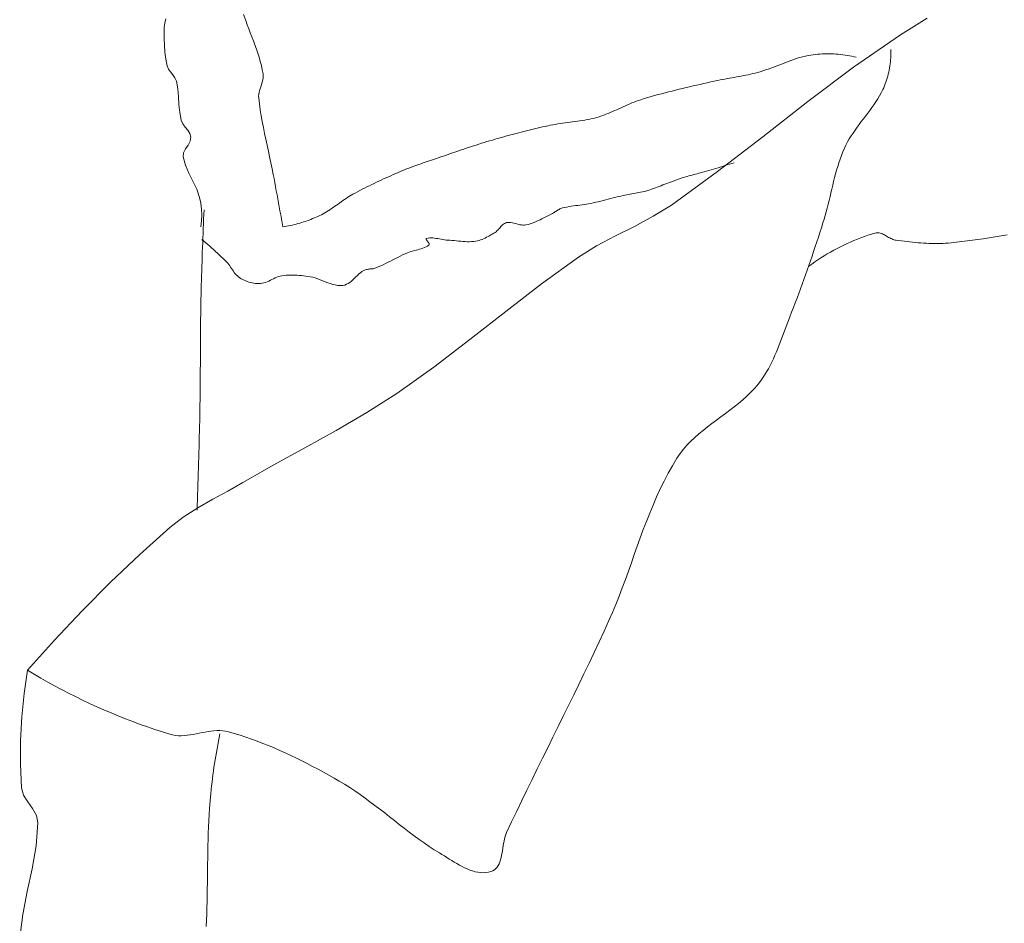
# Model space of a CAD drawing. Units: inches. Extents: x -36302355 to 648, y -221479757 to 75.
# Tile 25 of 37: x 192 to 220, y -218 to -192. Entities that reach past the tile are written whole.
import ezdxf

# ---------------------------------------------------------------- set-up
doc = ezdxf.new("R2010")
doc.units = ezdxf.units.IN
doc.header["$MEASUREMENT"] = 0
doc.layers.add('A-FURN', color=8, linetype='Continuous', lineweight=13)

# ---------------------------------------------------------------- blocks, each defined once
blk = doc.blocks.new('BED-DOUBLE')
for p, q in [((4.097, 63.43), (4.117, 63.548)), ((6.36, 63.496), (6.296, 63.67)), ((6.401, 63.383), (6.36, 63.496)), ((25.45, 63.569), (24.695, 63.097)), ((4.072, 63.192), (4.078, 63.311)), ((4.076, 62.999), (4.072, 63.192)), ((4.078, 63.311), (4.097, 63.43)), ((6.444, 63.269), (6.401, 63.383)), ((6.488, 63.156), (6.444, 63.269)), ((6.531, 63.043), (6.488, 63.156)), ((4.083, 62.806), (4.076, 62.999)), ((6.574, 62.929), (6.531, 63.043)), ((6.616, 62.816), (6.574, 62.929)), ((24.695, 63.097), (23.379, 62.192)), ((4.096, 62.613), (4.083, 62.806)), ((4.119, 62.421), (4.096, 62.613)), ((6.657, 62.702), (6.616, 62.816)), ((6.696, 62.587), (6.657, 62.702)), ((24.428, 62.63), (24.425, 62.688)), ((24.428, 62.573), (24.428, 62.63)), ((4.157, 62.233), (4.119, 62.421)), ((6.733, 62.472), (6.696, 62.587)), ((6.767, 62.356), (6.733, 62.472)), ((6.797, 62.24), (6.767, 62.356)), ((21.511, 62.338), (21.437, 62.31)), ((21.585, 62.366), (21.511, 62.338)), ((21.659, 62.392), (21.585, 62.366)), ((21.733, 62.418), (21.659, 62.392)), ((21.808, 62.442), (21.733, 62.418)), ((21.883, 62.464), (21.808, 62.442)), ((21.958, 62.485), (21.883, 62.464)), ((22.034, 62.503), (21.958, 62.485)), ((22.111, 62.519), (22.034, 62.503)), ((22.188, 62.532), (22.111, 62.519)), ((22.251, 62.541), (22.188, 62.532)), ((22.315, 62.549), (22.251, 62.541)), ((22.378, 62.555), (22.315, 62.549)), ((22.442, 62.561), (22.378, 62.555)), ((22.506, 62.564), (22.442, 62.561)), ((22.57, 62.567), (22.506, 62.564)), ((22.635, 62.568), (22.57, 62.567)), ((22.699, 62.568), (22.635, 62.568)), ((22.763, 62.567), (22.699, 62.568)), ((22.828, 62.565), (22.763, 62.567)), ((22.892, 62.561), (22.828, 62.565)), ((22.956, 62.556), (22.892, 62.561)), ((23.02, 62.55), (22.956, 62.556)), ((23.084, 62.542), (23.02, 62.55)), ((23.148, 62.533), (23.084, 62.542)), ((23.211, 62.523), (23.148, 62.533)), ((23.274, 62.512), (23.211, 62.523)), ((23.337, 62.499), (23.274, 62.512)), ((23.399, 62.485), (23.337, 62.499)), ((23.461, 62.47), (23.399, 62.485)), ((24.41, 62.285), (24.417, 62.342)), ((24.417, 62.342), (24.422, 62.4)), ((24.422, 62.4), (24.425, 62.458)), ((24.425, 62.458), (24.428, 62.515)), ((24.428, 62.515), (24.428, 62.573)), ((4.195, 62.142), (4.157, 62.233)), ((4.253, 62.059), (4.195, 62.142)), ((4.318, 61.979), (4.253, 62.059)), ((6.824, 62.122), (6.797, 62.24)), ((6.846, 62.004), (6.824, 62.122)), ((20.771, 62.067), (20.695, 62.046)), ((20.846, 62.09), (20.771, 62.067)), ((20.921, 62.115), (20.846, 62.09)), ((20.995, 62.141), (20.921, 62.115)), ((21.069, 62.168), (20.995, 62.141)), ((21.143, 62.196), (21.069, 62.168)), ((21.217, 62.224), (21.143, 62.196)), ((21.29, 62.253), (21.217, 62.224)), ((21.364, 62.282), (21.29, 62.253)), ((21.437, 62.31), (21.364, 62.282)), ((23.379, 62.192), (22.102, 61.232)), ((24.358, 62), (24.371, 62.056)), ((24.371, 62.056), (24.383, 62.113)), ((24.383, 62.113), (24.394, 62.17)), ((24.394, 62.17), (24.403, 62.227)), ((24.403, 62.227), (24.41, 62.285)), ((4.377, 61.896), (4.318, 61.979)), ((4.416, 61.805), (4.377, 61.896)), ((4.456, 61.588), (4.416, 61.805)), ((6.815, 61.746), (6.83, 61.798)), ((6.83, 61.798), (6.842, 61.849)), ((6.842, 61.849), (6.849, 61.9)), ((6.851, 61.952), (6.846, 62.004)), ((6.849, 61.9), (6.851, 61.952)), ((19.383, 61.781), (19.285, 61.759)), ((19.449, 61.796), (19.383, 61.781)), ((19.514, 61.81), (19.449, 61.796)), ((19.58, 61.824), (19.514, 61.81)), ((19.645, 61.837), (19.58, 61.824)), ((19.711, 61.849), (19.645, 61.837)), ((19.777, 61.862), (19.711, 61.849)), ((19.843, 61.873), (19.777, 61.862)), ((19.909, 61.885), (19.843, 61.873)), ((19.975, 61.897), (19.909, 61.885)), ((20.041, 61.909), (19.975, 61.897)), ((20.107, 61.92), (20.041, 61.909)), ((20.172, 61.932), (20.107, 61.92)), ((20.238, 61.945), (20.172, 61.932)), ((20.304, 61.957), (20.238, 61.945)), ((20.37, 61.97), (20.304, 61.957)), ((20.435, 61.984), (20.37, 61.97)), ((20.5, 61.998), (20.435, 61.984)), ((20.566, 62.013), (20.5, 61.998)), ((20.631, 62.029), (20.566, 62.013)), ((20.695, 62.046), (20.631, 62.029)), ((24.272, 61.724), (24.292, 61.778)), ((24.292, 61.778), (24.31, 61.833)), ((24.31, 61.833), (24.327, 61.888)), ((24.327, 61.888), (24.343, 61.944)), ((24.343, 61.944), (24.358, 62)), ((4.476, 61.367), (4.456, 61.588)), ((6.735, 61.489), (6.748, 61.541)), ((6.748, 61.541), (6.764, 61.592)), ((6.764, 61.592), (6.781, 61.644)), ((6.781, 61.644), (6.799, 61.695)), ((6.799, 61.695), (6.815, 61.746)), ((18.204, 61.502), (18.106, 61.477)), ((18.302, 61.526), (18.204, 61.502)), ((18.4, 61.551), (18.302, 61.526)), ((18.498, 61.574), (18.4, 61.551)), ((18.596, 61.598), (18.498, 61.574)), ((18.695, 61.621), (18.596, 61.598)), ((18.793, 61.645), (18.695, 61.621)), ((18.891, 61.667), (18.793, 61.645)), ((18.99, 61.69), (18.891, 61.667)), ((19.088, 61.713), (18.99, 61.69)), ((19.187, 61.736), (19.088, 61.713)), ((19.285, 61.759), (19.187, 61.736)), ((24.161, 61.478), (24.205, 61.565)), ((24.205, 61.565), (24.228, 61.618)), ((24.228, 61.618), (24.251, 61.67)), ((24.251, 61.67), (24.272, 61.724)), ((4.49, 61.145), (4.476, 61.367)), ((6.721, 61.386), (6.725, 61.438)), ((6.723, 61.334), (6.721, 61.386)), ((6.742, 61.167), (6.723, 61.334)), ((6.725, 61.438), (6.735, 61.489)), ((17.3, 61.242), (17.238, 61.218)), ((17.363, 61.264), (17.3, 61.242)), ((17.426, 61.284), (17.363, 61.264)), ((17.522, 61.314), (17.426, 61.284)), ((17.619, 61.343), (17.522, 61.314)), ((17.716, 61.371), (17.619, 61.343)), ((17.813, 61.398), (17.716, 61.371)), ((17.911, 61.425), (17.813, 61.398)), ((18.008, 61.451), (17.911, 61.425)), ((18.106, 61.477), (18.008, 61.451)), ((22.102, 61.232), (20.841, 60.248)), ((23.957, 61.144), (24.012, 61.225)), ((24.012, 61.225), (24.064, 61.308)), ((24.064, 61.308), (24.114, 61.392)), ((24.114, 61.392), (24.161, 61.478)), ((4.51, 60.924), (4.49, 61.145)), ((6.765, 61), (6.742, 61.167)), ((6.792, 60.835), (6.765, 61)), ((16.631, 60.95), (16.57, 60.924)), ((16.692, 60.977), (16.631, 60.95)), ((16.752, 61.004), (16.692, 60.977)), ((16.813, 61.032), (16.752, 61.004)), ((16.873, 61.06), (16.813, 61.032)), ((16.934, 61.087), (16.873, 61.06)), ((16.994, 61.115), (16.934, 61.087)), ((17.055, 61.142), (16.994, 61.115)), ((17.116, 61.168), (17.055, 61.142)), ((17.177, 61.194), (17.116, 61.168)), ((17.238, 61.218), (17.177, 61.194)), ((23.783, 60.905), (23.842, 60.984)), ((23.842, 60.984), (23.9, 61.063)), ((23.9, 61.063), (23.957, 61.144)), ((4.551, 60.707), (4.51, 60.924)), ((4.596, 60.607), (4.551, 60.707)), ((6.821, 60.669), (6.792, 60.835)), ((15.651, 60.68), (15.582, 60.67)), ((15.72, 60.69), (15.651, 60.68)), ((15.789, 60.701), (15.72, 60.69)), ((15.857, 60.713), (15.789, 60.701)), ((15.926, 60.726), (15.857, 60.713)), ((15.994, 60.739), (15.926, 60.726)), ((16.062, 60.754), (15.994, 60.739)), ((16.13, 60.771), (16.062, 60.754)), ((16.197, 60.789), (16.13, 60.771)), ((16.261, 60.808), (16.197, 60.789)), ((16.323, 60.828), (16.261, 60.808)), ((16.386, 60.85), (16.323, 60.828)), ((16.448, 60.874), (16.386, 60.85)), ((16.509, 60.898), (16.448, 60.874)), ((16.57, 60.924), (16.509, 60.898)), ((23.602, 60.669), (23.662, 60.748)), ((23.662, 60.748), (23.723, 60.826)), ((23.723, 60.826), (23.783, 60.905)), ((4.665, 60.516), (4.596, 60.607)), ((4.738, 60.428), (4.665, 60.516)), ((4.798, 60.335), (4.738, 60.428)), ((6.853, 60.504), (6.821, 60.669)), ((6.887, 60.34), (6.853, 60.504)), ((14.227, 60.416), (14.153, 60.397)), ((14.301, 60.434), (14.227, 60.416)), ((14.376, 60.452), (14.301, 60.434)), ((14.45, 60.47), (14.376, 60.452)), ((14.524, 60.487), (14.45, 60.47)), ((14.599, 60.504), (14.524, 60.487)), ((14.673, 60.521), (14.599, 60.504)), ((14.748, 60.538), (14.673, 60.521)), ((14.822, 60.554), (14.748, 60.538)), ((14.891, 60.568), (14.822, 60.554)), ((14.959, 60.581), (14.891, 60.568)), ((15.028, 60.593), (14.959, 60.581)), ((15.097, 60.604), (15.028, 60.593)), ((15.166, 60.614), (15.097, 60.604)), ((15.235, 60.624), (15.166, 60.614)), ((15.304, 60.633), (15.235, 60.624)), ((15.374, 60.642), (15.304, 60.633)), ((15.443, 60.652), (15.374, 60.642)), ((15.512, 60.661), (15.443, 60.652)), ((15.582, 60.67), (15.512, 60.661)), ((23.37, 60.351), (23.426, 60.431)), ((23.426, 60.431), (23.484, 60.511)), ((23.484, 60.511), (23.542, 60.59)), ((23.542, 60.59), (23.602, 60.669)), ((4.826, 60.233), (4.798, 60.335)), ((4.805, 60.119), (4.826, 60.233)), ((6.922, 60.175), (6.887, 60.34)), ((6.958, 60.011), (6.922, 60.175)), ((13.192, 60.132), (13.117, 60.109)), ((13.267, 60.154), (13.192, 60.132)), ((13.343, 60.176), (13.267, 60.154)), ((13.416, 60.198), (13.343, 60.176)), ((13.489, 60.219), (13.416, 60.198)), ((13.563, 60.239), (13.489, 60.219)), ((13.636, 60.26), (13.563, 60.239)), ((13.71, 60.28), (13.636, 60.26)), ((13.784, 60.3), (13.71, 60.28)), ((13.857, 60.32), (13.784, 60.3)), ((13.931, 60.34), (13.857, 60.32)), ((14.005, 60.359), (13.931, 60.34)), ((14.079, 60.378), (14.005, 60.359)), ((14.153, 60.397), (14.079, 60.378)), ((20.841, 60.248), (19.575, 59.272)), ((23.215, 60.101), (23.264, 60.186)), ((23.264, 60.186), (23.316, 60.269)), ((23.316, 60.269), (23.37, 60.351)), ((4.62, 59.798), (4.675, 59.905)), ((4.675, 59.905), (4.746, 60.011)), ((4.746, 60.011), (4.805, 60.119)), ((6.994, 59.846), (6.958, 60.011)), ((7.03, 59.682), (6.994, 59.846)), ((12.37, 59.867), (12.296, 59.842)), ((12.445, 59.892), (12.37, 59.867)), ((12.519, 59.917), (12.445, 59.892)), ((12.594, 59.942), (12.519, 59.917)), ((12.668, 59.967), (12.594, 59.942)), ((12.743, 59.991), (12.668, 59.967)), ((12.817, 60.015), (12.743, 59.991)), ((12.892, 60.039), (12.817, 60.015)), ((12.967, 60.063), (12.892, 60.039)), ((13.042, 60.086), (12.967, 60.063)), ((13.117, 60.109), (13.042, 60.086)), ((23.085, 59.826), (23.128, 59.926)), ((23.128, 59.926), (23.17, 60.015)), ((23.17, 60.015), (23.215, 60.101)), ((4.607, 59.685), (4.62, 59.798)), ((4.668, 59.449), (4.607, 59.685)), ((7.066, 59.517), (7.03, 59.682)), ((11.501, 59.572), (11.443, 59.553)), ((11.56, 59.592), (11.501, 59.572)), ((11.618, 59.612), (11.56, 59.592)), ((11.676, 59.631), (11.618, 59.612)), ((11.734, 59.651), (11.676, 59.631)), ((11.792, 59.671), (11.734, 59.651)), ((11.85, 59.69), (11.792, 59.671)), ((11.924, 59.716), (11.85, 59.69)), ((11.999, 59.741), (11.924, 59.716)), ((12.073, 59.766), (11.999, 59.741)), ((12.147, 59.792), (12.073, 59.766)), ((12.221, 59.817), (12.147, 59.792)), ((12.296, 59.842), (12.221, 59.817)), ((22.973, 59.521), (23.007, 59.623)), ((23.007, 59.623), (23.045, 59.725)), ((23.045, 59.725), (23.085, 59.826)), ((4.766, 59.224), (4.668, 59.449)), ((7.1, 59.353), (7.066, 59.517)), ((7.132, 59.188), (7.1, 59.353)), ((10.753, 59.298), (10.697, 59.275)), ((10.81, 59.321), (10.753, 59.298)), ((10.867, 59.344), (10.81, 59.321)), ((10.924, 59.366), (10.867, 59.344)), ((10.981, 59.388), (10.924, 59.366)), ((11.039, 59.41), (10.981, 59.388)), ((11.096, 59.431), (11.039, 59.41)), ((11.154, 59.452), (11.096, 59.431)), ((11.212, 59.472), (11.154, 59.452)), ((11.269, 59.493), (11.212, 59.472)), ((11.327, 59.513), (11.269, 59.493)), ((11.385, 59.533), (11.327, 59.513)), ((11.443, 59.553), (11.385, 59.533)), ((19.327, 59.302), (19.262, 59.283)), ((19.392, 59.321), (19.327, 59.302)), ((19.458, 59.341), (19.392, 59.321)), ((19.523, 59.36), (19.458, 59.341)), ((19.588, 59.379), (19.523, 59.36)), ((19.653, 59.399), (19.588, 59.379)), ((19.718, 59.418), (19.653, 59.399)), ((19.783, 59.438), (19.718, 59.418)), ((19.848, 59.458), (19.783, 59.438)), ((19.913, 59.478), (19.848, 59.458)), ((19.978, 59.498), (19.913, 59.478)), ((20.043, 59.518), (19.978, 59.498)), ((22.88, 59.208), (22.909, 59.313)), ((22.909, 59.313), (22.94, 59.417)), ((22.94, 59.417), (22.973, 59.521)), ((4.88, 59.003), (4.766, 59.224)), ((7.153, 59.075), (7.132, 59.188)), ((7.174, 58.962), (7.153, 59.075)), ((10.156, 59.035), (10.089, 59.004)), ((10.223, 59.066), (10.156, 59.035)), ((10.29, 59.097), (10.223, 59.066)), ((10.358, 59.127), (10.29, 59.097)), ((10.425, 59.157), (10.358, 59.127)), ((10.493, 59.187), (10.425, 59.157)), ((10.561, 59.216), (10.493, 59.187)), ((10.629, 59.246), (10.561, 59.216)), ((10.697, 59.275), (10.629, 59.246)), ((19.575, 59.272), (18.281, 58.335)), ((18.381, 59.024), (18.356, 59.015)), ((18.406, 59.033), (18.381, 59.024)), ((18.431, 59.043), (18.406, 59.033)), ((18.455, 59.052), (18.431, 59.043)), ((18.48, 59.061), (18.455, 59.052)), ((18.505, 59.07), (18.48, 59.061)), ((18.53, 59.078), (18.505, 59.07)), ((18.555, 59.086), (18.53, 59.078)), ((18.58, 59.094), (18.555, 59.086)), ((18.627, 59.108), (18.58, 59.094)), ((18.675, 59.122), (18.627, 59.108)), ((18.722, 59.135), (18.675, 59.122)), ((18.769, 59.149), (18.722, 59.135)), ((18.817, 59.161), (18.769, 59.149)), ((18.864, 59.174), (18.817, 59.161)), ((18.912, 59.187), (18.864, 59.174)), ((18.959, 59.199), (18.912, 59.187)), ((19.007, 59.212), (18.959, 59.199)), ((19.054, 59.225), (19.007, 59.212)), ((19.102, 59.238), (19.054, 59.225)), ((19.149, 59.251), (19.102, 59.238)), ((19.197, 59.264), (19.149, 59.251)), ((19.262, 59.283), (19.197, 59.264)), ((22.826, 58.996), (22.852, 59.102)), ((22.852, 59.102), (22.88, 59.208)), ((4.988, 58.78), (4.88, 59.003)), ((5.069, 58.548), (4.988, 58.78)), ((7.195, 58.849), (7.174, 58.962)), ((7.216, 58.737), (7.195, 58.849)), ((9.624, 58.776), (9.559, 58.741)), ((9.69, 58.809), (9.624, 58.776)), ((9.756, 58.842), (9.69, 58.809)), ((9.822, 58.875), (9.756, 58.842)), ((9.889, 58.908), (9.822, 58.875)), ((9.955, 58.94), (9.889, 58.908)), ((10.022, 58.972), (9.955, 58.94)), ((10.089, 59.004), (10.022, 58.972)), ((17.62, 58.744), (17.566, 58.728)), ((17.674, 58.761), (17.62, 58.744)), ((17.727, 58.779), (17.674, 58.761)), ((17.781, 58.798), (17.727, 58.779)), ((17.834, 58.817), (17.781, 58.798)), ((17.887, 58.837), (17.834, 58.817)), ((17.94, 58.857), (17.887, 58.837)), ((17.993, 58.877), (17.94, 58.857)), ((18.046, 58.898), (17.993, 58.877)), ((18.098, 58.918), (18.046, 58.898)), ((18.151, 58.938), (18.098, 58.918)), ((18.204, 58.958), (18.151, 58.938)), ((18.257, 58.978), (18.204, 58.958)), ((18.282, 58.987), (18.257, 58.978)), ((18.307, 58.996), (18.282, 58.987)), ((18.332, 59.005), (18.307, 58.996)), ((18.356, 59.015), (18.332, 59.005)), ((22.75, 58.678), (22.775, 58.784)), ((22.775, 58.784), (22.8, 58.89)), ((22.8, 58.89), (22.826, 58.996)), ((5.103, 58.387), (5.069, 58.548)), ((7.236, 58.624), (7.216, 58.737)), ((7.257, 58.511), (7.236, 58.624)), ((7.278, 58.398), (7.257, 58.511)), ((9.128, 58.491), (9.082, 58.46)), ((9.174, 58.522), (9.128, 58.491)), ((9.22, 58.553), (9.174, 58.522)), ((9.267, 58.582), (9.22, 58.553)), ((9.315, 58.61), (9.267, 58.582)), ((9.363, 58.637), (9.315, 58.61)), ((9.428, 58.672), (9.363, 58.637)), ((9.493, 58.707), (9.428, 58.672)), ((9.559, 58.741), (9.493, 58.707)), ((16.443, 58.481), (16.374, 58.463)), ((16.513, 58.5), (16.443, 58.481)), ((16.583, 58.518), (16.513, 58.5)), ((16.653, 58.536), (16.583, 58.518)), ((16.723, 58.554), (16.653, 58.536)), ((16.792, 58.571), (16.723, 58.554)), ((16.862, 58.588), (16.792, 58.571)), ((16.933, 58.604), (16.862, 58.588)), ((16.981, 58.615), (16.933, 58.604)), ((17.03, 58.624), (16.981, 58.615)), ((17.079, 58.633), (17.03, 58.624)), ((17.128, 58.642), (17.079, 58.633)), ((17.177, 58.65), (17.128, 58.642)), ((17.226, 58.658), (17.177, 58.65)), ((17.275, 58.666), (17.226, 58.658)), ((17.324, 58.675), (17.275, 58.666)), ((17.372, 58.684), (17.324, 58.675)), ((17.421, 58.693), (17.372, 58.684)), ((17.469, 58.704), (17.421, 58.693)), ((17.518, 58.716), (17.469, 58.704)), ((17.566, 58.728), (17.518, 58.716)), ((22.699, 58.465), (22.725, 58.571)), ((22.725, 58.571), (22.75, 58.678)), ((5.123, 58.222), (5.103, 58.387)), ((5.13, 58.056), (5.123, 58.222)), ((5.187, 58.07), (5.194, 58.202)), ((7.298, 58.285), (7.278, 58.398)), ((7.319, 58.172), (7.298, 58.285)), ((8.719, 58.205), (8.672, 58.175)), ((8.765, 58.236), (8.719, 58.205)), ((8.81, 58.267), (8.765, 58.236)), ((8.856, 58.299), (8.81, 58.267)), ((8.901, 58.331), (8.856, 58.299)), ((8.946, 58.364), (8.901, 58.331)), ((8.991, 58.396), (8.946, 58.364)), ((9.037, 58.428), (8.991, 58.396)), ((9.082, 58.46), (9.037, 58.428)), ((15.114, 58.199), (15.091, 58.186)), ((15.137, 58.213), (15.114, 58.199)), ((15.161, 58.225), (15.137, 58.213)), ((15.185, 58.236), (15.161, 58.225)), ((15.21, 58.245), (15.185, 58.236)), ((15.235, 58.253), (15.21, 58.245)), ((15.295, 58.267), (15.235, 58.253)), ((15.355, 58.28), (15.295, 58.267)), ((15.415, 58.291), (15.355, 58.28)), ((15.476, 58.301), (15.415, 58.291)), ((15.536, 58.31), (15.476, 58.301)), ((15.597, 58.318), (15.536, 58.31)), ((15.658, 58.326), (15.597, 58.318)), ((15.719, 58.333), (15.658, 58.326)), ((15.78, 58.341), (15.719, 58.333)), ((15.841, 58.35), (15.78, 58.341)), ((15.902, 58.359), (15.841, 58.35)), ((15.963, 58.369), (15.902, 58.359)), ((16.023, 58.381), (15.963, 58.369)), ((16.093, 58.396), (16.023, 58.381)), ((16.164, 58.412), (16.093, 58.396)), ((16.234, 58.428), (16.164, 58.412)), ((16.304, 58.446), (16.234, 58.428)), ((16.374, 58.463), (16.304, 58.446)), ((18.281, 58.335), (17.775, 58.02)), ((22.619, 58.147), (22.647, 58.252)), ((22.647, 58.252), (22.674, 58.358)), ((22.674, 58.358), (22.699, 58.465)), ((5.124, 57.891), (5.13, 58.056)), ((5.176, 57.807), (5.181, 57.938)), ((5.181, 57.938), (5.187, 58.07)), ((7.339, 58.06), (7.319, 58.172)), ((7.36, 57.947), (7.339, 58.06)), ((7.38, 57.834), (7.36, 57.947)), ((8.132, 57.916), (8.081, 57.897)), ((8.183, 57.935), (8.132, 57.916)), ((8.233, 57.955), (8.183, 57.935)), ((8.283, 57.975), (8.233, 57.955)), ((8.333, 57.996), (8.283, 57.975)), ((8.382, 58.018), (8.333, 57.996)), ((8.431, 58.041), (8.382, 58.018)), ((8.481, 58.065), (8.431, 58.041)), ((8.53, 58.09), (8.481, 58.065)), ((8.578, 58.117), (8.53, 58.09)), ((8.626, 58.146), (8.578, 58.117)), ((8.672, 58.175), (8.626, 58.146)), ((14.603, 57.925), (14.548, 57.899)), ((14.657, 57.953), (14.603, 57.925)), ((14.711, 57.981), (14.657, 57.953)), ((14.766, 58.009), (14.711, 57.981)), ((14.82, 58.037), (14.766, 58.009)), ((14.874, 58.064), (14.82, 58.037)), ((14.929, 58.09), (14.874, 58.064)), ((14.953, 58.102), (14.929, 58.09)), ((14.976, 58.115), (14.953, 58.102)), ((15, 58.128), (14.976, 58.115)), ((15.022, 58.143), (15, 58.128)), ((15.045, 58.157), (15.022, 58.143)), ((15.068, 58.171), (15.045, 58.157)), ((15.091, 58.186), (15.068, 58.171)), ((17.775, 58.02), (17.248, 57.739)), ((22.527, 57.833), (22.56, 57.937)), ((22.56, 57.937), (22.59, 58.042)), ((22.59, 58.042), (22.619, 58.147)), ((5.104, 57.727), (5.124, 57.891)), ((5.164, 57.543), (5.17, 57.675)), ((5.17, 57.675), (5.176, 57.807)), ((7.4, 57.721), (7.38, 57.834)), ((7.453, 57.73), (7.4, 57.721)), ((7.506, 57.74), (7.453, 57.73)), ((7.559, 57.751), (7.506, 57.74)), ((7.612, 57.762), (7.559, 57.751)), ((7.665, 57.774), (7.612, 57.762)), ((7.718, 57.787), (7.665, 57.774)), ((7.77, 57.801), (7.718, 57.787)), ((7.823, 57.815), (7.77, 57.801)), ((7.875, 57.83), (7.823, 57.815)), ((7.927, 57.846), (7.875, 57.83)), ((7.978, 57.862), (7.927, 57.846)), ((8.03, 57.879), (7.978, 57.862)), ((8.081, 57.897), (8.03, 57.879)), ((13.442, 57.658), (13.419, 57.633)), ((13.464, 57.683), (13.442, 57.658)), ((13.486, 57.709), (13.464, 57.683)), ((13.509, 57.734), (13.486, 57.709)), ((13.531, 57.758), (13.509, 57.734)), ((13.554, 57.781), (13.531, 57.758)), ((13.579, 57.801), (13.554, 57.781)), ((13.605, 57.819), (13.579, 57.801)), ((13.633, 57.832), (13.605, 57.819)), ((13.663, 57.842), (13.633, 57.832)), ((13.704, 57.849), (13.663, 57.842)), ((13.746, 57.85), (13.704, 57.849)), ((13.787, 57.847), (13.746, 57.85)), ((13.829, 57.84), (13.787, 57.847)), ((13.871, 57.83), (13.829, 57.84)), ((13.914, 57.819), (13.871, 57.83)), ((13.956, 57.807), (13.914, 57.819)), ((13.998, 57.795), (13.956, 57.807)), ((14.04, 57.785), (13.998, 57.795)), ((14.082, 57.778), (14.04, 57.785)), ((14.124, 57.773), (14.082, 57.778)), ((14.166, 57.773), (14.124, 57.773)), ((14.208, 57.778), (14.166, 57.773)), ((14.266, 57.791), (14.208, 57.778)), ((14.324, 57.808), (14.266, 57.791)), ((14.381, 57.827), (14.324, 57.808)), ((14.437, 57.849), (14.381, 57.827)), ((14.493, 57.873), (14.437, 57.849)), ((14.548, 57.899), (14.493, 57.873)), ((17.248, 57.739), (16.714, 57.469)), ((22.441, 57.568), (22.484, 57.701)), ((22.484, 57.701), (22.527, 57.833)), ((5.185, 57.325), (5.129, 57.371)), ((5.154, 57.279), (5.159, 57.411)), ((5.159, 57.411), (5.164, 57.543)), ((11.414, 57.394), (11.411, 57.385)), ((11.411, 57.385), (11.414, 57.373)), ((11.425, 57.4), (11.414, 57.394)), ((11.414, 57.373), (11.422, 57.359)), ((11.469, 57.409), (11.425, 57.4)), ((11.514, 57.414), (11.469, 57.409)), ((11.559, 57.415), (11.514, 57.414)), ((11.604, 57.413), (11.559, 57.415)), ((11.649, 57.409), (11.604, 57.413)), ((11.695, 57.403), (11.649, 57.409)), ((11.741, 57.395), (11.695, 57.403)), ((11.787, 57.386), (11.741, 57.395)), ((11.832, 57.378), (11.787, 57.386)), ((11.878, 57.369), (11.832, 57.378)), ((11.924, 57.362), (11.878, 57.369)), ((12.981, 57.375), (12.939, 57.359)), ((13.023, 57.392), (12.981, 57.375)), ((13.065, 57.412), (13.023, 57.392)), ((13.106, 57.432), (13.065, 57.412)), ((13.146, 57.454), (13.106, 57.432)), ((13.186, 57.477), (13.146, 57.454)), ((13.226, 57.5), (13.186, 57.477)), ((13.266, 57.523), (13.226, 57.5)), ((13.305, 57.547), (13.266, 57.523)), ((13.344, 57.571), (13.305, 57.547)), ((13.371, 57.589), (13.344, 57.571)), ((13.396, 57.61), (13.371, 57.589)), ((13.419, 57.633), (13.396, 57.61)), ((16.714, 57.469), (16.186, 57.189)), ((22.354, 57.303), (22.398, 57.436)), ((22.398, 57.436), (22.441, 57.568)), ((23.493, 57.381), (23.396, 57.341)), ((23.59, 57.418), (23.493, 57.381)), ((23.688, 57.454), (23.59, 57.418)), ((23.786, 57.488), (23.688, 57.454)), ((23.885, 57.52), (23.786, 57.488)), ((23.984, 57.551), (23.885, 57.52)), ((24.014, 57.558), (23.984, 57.551)), ((24.044, 57.56), (24.014, 57.558)), ((24.074, 57.559), (24.044, 57.56)), ((24.103, 57.555), (24.074, 57.559)), ((24.133, 57.548), (24.103, 57.555)), ((24.162, 57.538), (24.133, 57.548)), ((24.191, 57.526), (24.162, 57.538)), ((24.22, 57.513), (24.191, 57.526)), ((24.25, 57.498), (24.22, 57.513)), ((24.279, 57.482), (24.25, 57.498)), ((24.308, 57.465), (24.279, 57.482)), ((24.338, 57.448), (24.308, 57.465)), ((24.367, 57.431), (24.338, 57.448)), ((24.397, 57.415), (24.367, 57.431)), ((24.426, 57.399), (24.397, 57.415)), ((24.456, 57.385), (24.426, 57.399)), ((24.487, 57.372), (24.456, 57.385)), ((24.517, 57.362), (24.487, 57.372)), ((27.018, 57.393), (26.793, 57.36)), ((27.243, 57.428), (27.018, 57.393)), ((27.467, 57.465), (27.243, 57.428)), ((27.691, 57.503), (27.467, 57.465)), ((5.144, 57.015), (5.149, 57.147)), ((5.149, 57.147), (5.154, 57.279)), ((5.24, 57.278), (5.185, 57.325)), ((5.295, 57.231), (5.24, 57.278)), ((5.35, 57.183), (5.295, 57.231)), ((5.405, 57.135), (5.35, 57.183)), ((5.459, 57.087), (5.405, 57.135)), ((11.225, 57.098), (11.177, 57.085)), ((11.273, 57.111), (11.225, 57.098)), ((11.319, 57.127), (11.273, 57.111)), ((11.365, 57.144), (11.319, 57.127)), ((11.409, 57.165), (11.365, 57.144)), ((11.451, 57.188), (11.409, 57.165)), ((11.422, 57.359), (11.433, 57.343)), ((11.433, 57.343), (11.447, 57.325)), ((11.447, 57.325), (11.461, 57.307)), ((11.491, 57.216), (11.451, 57.188)), ((11.461, 57.307), (11.475, 57.289)), ((11.475, 57.289), (11.487, 57.271)), ((11.487, 57.271), (11.496, 57.255)), ((11.5, 57.226), (11.491, 57.216)), ((11.496, 57.255), (11.501, 57.239)), ((11.501, 57.239), (11.5, 57.226)), ((11.97, 57.356), (11.924, 57.362)), ((12.015, 57.352), (11.97, 57.356)), ((12.076, 57.348), (12.015, 57.352)), ((12.137, 57.343), (12.076, 57.348)), ((12.198, 57.338), (12.137, 57.343)), ((12.26, 57.331), (12.198, 57.338)), ((12.321, 57.325), (12.26, 57.331)), ((12.382, 57.32), (12.321, 57.325)), ((12.443, 57.315), (12.382, 57.32)), ((12.504, 57.311), (12.443, 57.315)), ((12.565, 57.309), (12.504, 57.311)), ((12.626, 57.309), (12.565, 57.309)), ((12.686, 57.312), (12.626, 57.309)), ((12.747, 57.317), (12.686, 57.312)), ((12.807, 57.325), (12.747, 57.317)), ((12.852, 57.334), (12.807, 57.325)), ((12.895, 57.345), (12.852, 57.334)), ((12.939, 57.359), (12.895, 57.345)), ((16.186, 57.189), (15.68, 56.875)), ((22.266, 57.039), (22.31, 57.171)), ((22.31, 57.171), (22.354, 57.303)), ((22.924, 57.12), (22.831, 57.07)), ((23.017, 57.167), (22.924, 57.12)), ((23.11, 57.213), (23.017, 57.167)), ((23.205, 57.258), (23.11, 57.213)), ((23.3, 57.3), (23.205, 57.258)), ((23.396, 57.341), (23.3, 57.3)), ((24.548, 57.354), (24.517, 57.362)), ((24.579, 57.348), (24.548, 57.354)), ((24.655, 57.338), (24.579, 57.348)), ((24.732, 57.329), (24.655, 57.338)), ((24.808, 57.32), (24.732, 57.329)), ((24.885, 57.311), (24.808, 57.32)), ((24.962, 57.302), (24.885, 57.311)), ((25.039, 57.294), (24.962, 57.302)), ((25.116, 57.287), (25.039, 57.294)), ((25.193, 57.28), (25.116, 57.287)), ((25.27, 57.274), (25.193, 57.28)), ((25.347, 57.269), (25.27, 57.274)), ((25.424, 57.264), (25.347, 57.269)), ((25.501, 57.261), (25.424, 57.264)), ((25.578, 57.258), (25.501, 57.261)), ((25.655, 57.257), (25.578, 57.258)), ((25.732, 57.257), (25.655, 57.257)), ((25.809, 57.258), (25.732, 57.257)), ((25.886, 57.261), (25.809, 57.258)), ((25.963, 57.265), (25.886, 57.261)), ((26.039, 57.27), (25.963, 57.265)), ((26.116, 57.277), (26.039, 57.27)), ((26.342, 57.302), (26.116, 57.277)), ((26.568, 57.329), (26.342, 57.302)), ((26.793, 57.36), (26.568, 57.329)), ((5.135, 56.751), (5.139, 56.883)), ((5.139, 56.883), (5.144, 57.015)), ((5.513, 57.038), (5.459, 57.087)), ((5.566, 56.989), (5.513, 57.038)), ((5.619, 56.939), (5.566, 56.989)), ((5.671, 56.889), (5.619, 56.939)), ((5.723, 56.839), (5.671, 56.889)), ((5.775, 56.788), (5.723, 56.839)), ((10.55, 56.836), (10.482, 56.801)), ((10.617, 56.87), (10.55, 56.836)), ((10.685, 56.904), (10.617, 56.87)), ((10.754, 56.937), (10.685, 56.904)), ((10.822, 56.969), (10.754, 56.937)), ((10.892, 56.999), (10.822, 56.969)), ((10.937, 57.017), (10.892, 56.999)), ((10.984, 57.033), (10.937, 57.017)), ((11.032, 57.047), (10.984, 57.033)), ((11.08, 57.06), (11.032, 57.047)), ((11.129, 57.073), (11.08, 57.06)), ((11.177, 57.085), (11.129, 57.073)), ((15.68, 56.875), (14.648, 56.132)), ((22.177, 56.774), (22.221, 56.906)), ((22.221, 56.906), (22.266, 57.039)), ((22.472, 56.858), (22.385, 56.801)), ((22.561, 56.913), (22.472, 56.858)), ((22.65, 56.967), (22.561, 56.913)), ((22.74, 57.02), (22.65, 56.967)), ((22.831, 57.07), (22.74, 57.02)), ((5.127, 56.487), (5.131, 56.619)), ((5.131, 56.619), (5.135, 56.751)), ((5.826, 56.736), (5.775, 56.788)), ((5.856, 56.704), (5.826, 56.736)), ((5.885, 56.67), (5.856, 56.704)), ((5.911, 56.634), (5.885, 56.67)), ((5.937, 56.597), (5.911, 56.634)), ((5.962, 56.559), (5.937, 56.597)), ((5.987, 56.522), (5.962, 56.559)), ((9.79, 56.539), (9.764, 56.535)), ((9.817, 56.542), (9.79, 56.539)), ((9.844, 56.545), (9.817, 56.542)), ((9.872, 56.547), (9.844, 56.545)), ((9.899, 56.55), (9.872, 56.547)), ((9.925, 56.554), (9.899, 56.55)), ((9.952, 56.559), (9.925, 56.554)), ((9.977, 56.566), (9.952, 56.559)), ((10.003, 56.574), (9.977, 56.566)), ((10.073, 56.604), (10.003, 56.574)), ((10.142, 56.634), (10.073, 56.604)), ((10.211, 56.666), (10.142, 56.634)), ((10.279, 56.699), (10.211, 56.666)), ((10.347, 56.733), (10.279, 56.699)), ((10.414, 56.767), (10.347, 56.733)), ((10.482, 56.801), (10.414, 56.767)), ((22.086, 56.511), (22.131, 56.643)), ((22.214, 56.683), (22.13, 56.622)), ((22.131, 56.643), (22.177, 56.774)), ((22.299, 56.743), (22.214, 56.683)), ((22.385, 56.801), (22.299, 56.743)), ((5.119, 56.223), (5.123, 56.355)), ((5.123, 56.355), (5.127, 56.487)), ((6.013, 56.485), (5.987, 56.522)), ((6.039, 56.449), (6.013, 56.485)), ((6.066, 56.414), (6.039, 56.449)), ((6.095, 56.38), (6.066, 56.414)), ((6.125, 56.349), (6.095, 56.38)), ((6.158, 56.321), (6.125, 56.349)), ((6.194, 56.296), (6.158, 56.321)), ((6.234, 56.272), (6.194, 56.296)), ((6.274, 56.25), (6.234, 56.272)), ((7.139, 56.274), (7.094, 56.252)), ((7.184, 56.296), (7.139, 56.274)), ((7.23, 56.316), (7.184, 56.296)), ((7.276, 56.333), (7.23, 56.316)), ((7.323, 56.346), (7.276, 56.333)), ((7.371, 56.355), (7.323, 56.346)), ((7.432, 56.362), (7.371, 56.355)), ((7.492, 56.368), (7.432, 56.362)), ((7.553, 56.371), (7.492, 56.368)), ((7.614, 56.373), (7.553, 56.371)), ((7.676, 56.373), (7.614, 56.373)), ((7.737, 56.371), (7.676, 56.373)), ((7.798, 56.369), (7.737, 56.371)), ((7.859, 56.365), (7.798, 56.369)), ((7.92, 56.359), (7.859, 56.365)), ((7.981, 56.353), (7.92, 56.359)), ((8.042, 56.345), (7.981, 56.353)), ((8.103, 56.337), (8.042, 56.345)), ((8.163, 56.328), (8.103, 56.337)), ((8.235, 56.314), (8.163, 56.328)), ((8.306, 56.294), (8.235, 56.314)), ((8.377, 56.271), (8.306, 56.294)), ((8.448, 56.244), (8.377, 56.271)), ((9.404, 56.284), (9.363, 56.244)), ((9.445, 56.325), (9.404, 56.284)), ((9.486, 56.366), (9.445, 56.325)), ((9.528, 56.405), (9.486, 56.366)), ((9.571, 56.442), (9.528, 56.405)), ((9.616, 56.476), (9.571, 56.442)), ((9.663, 56.504), (9.616, 56.476)), ((9.687, 56.515), (9.663, 56.504)), ((9.712, 56.524), (9.687, 56.515)), ((9.738, 56.53), (9.712, 56.524)), ((9.764, 56.535), (9.738, 56.53)), ((21.993, 56.248), (22.039, 56.379)), ((22.039, 56.379), (22.086, 56.511)), ((5.112, 55.959), (5.115, 56.091)), ((5.115, 56.091), (5.119, 56.223)), ((6.317, 56.229), (6.274, 56.25)), ((6.36, 56.211), (6.317, 56.229)), ((6.404, 56.195), (6.36, 56.211)), ((6.449, 56.18), (6.404, 56.195)), ((6.494, 56.168), (6.449, 56.18)), ((6.54, 56.157), (6.494, 56.168)), ((6.586, 56.149), (6.54, 56.157)), ((6.633, 56.143), (6.586, 56.149)), ((6.679, 56.139), (6.633, 56.143)), ((6.725, 56.138), (6.679, 56.139)), ((6.772, 56.139), (6.725, 56.138)), ((6.82, 56.144), (6.772, 56.139)), ((6.867, 56.155), (6.82, 56.144)), ((6.914, 56.169), (6.867, 56.155)), ((6.959, 56.187), (6.914, 56.169)), ((7.005, 56.207), (6.959, 56.187)), ((7.05, 56.229), (7.005, 56.207)), ((7.094, 56.252), (7.05, 56.229)), ((8.518, 56.217), (8.448, 56.244)), ((8.588, 56.189), (8.518, 56.217)), ((8.658, 56.162), (8.588, 56.189)), ((8.728, 56.137), (8.658, 56.162)), ((8.798, 56.115), (8.728, 56.137)), ((8.869, 56.098), (8.798, 56.115)), ((8.94, 56.087), (8.869, 56.098)), ((9.011, 56.083), (8.94, 56.087)), ((9.084, 56.087), (9.011, 56.083)), ((9.137, 56.097), (9.084, 56.087)), ((9.186, 56.116), (9.137, 56.097)), ((9.233, 56.141), (9.186, 56.116)), ((9.278, 56.171), (9.233, 56.141)), ((9.321, 56.206), (9.278, 56.171)), ((9.363, 56.244), (9.321, 56.206)), ((14.648, 56.132), (13.641, 55.355)), ((21.85, 55.855), (21.898, 55.986)), ((21.898, 55.986), (21.946, 56.117)), ((21.946, 56.117), (21.993, 56.248)), ((5.106, 55.695), (5.109, 55.827)), ((5.109, 55.827), (5.112, 55.959)), ((21.751, 55.594), (21.801, 55.724)), ((21.801, 55.724), (21.85, 55.855)), ((5.1, 55.422), (5.103, 55.563)), ((5.103, 55.563), (5.106, 55.695)), ((21.65, 55.334), (21.701, 55.464)), ((21.701, 55.464), (21.751, 55.594)), ((5.096, 55.14), (5.098, 55.281)), ((5.098, 55.281), (5.1, 55.422)), ((13.641, 55.355), (12.64, 54.568)), ((21.56, 55.108), (21.599, 55.205)), ((21.599, 55.205), (21.65, 55.334)), ((5.093, 54.857), (5.094, 54.999)), ((5.094, 54.999), (5.096, 55.14)), ((21.449, 54.814), (21.486, 54.912)), ((21.486, 54.912), (21.523, 55.01)), ((21.523, 55.01), (21.56, 55.108)), ((5.091, 54.575), (5.092, 54.716)), ((5.092, 54.716), (5.093, 54.857)), ((21.338, 54.518), (21.375, 54.617)), ((21.375, 54.617), (21.412, 54.715)), ((21.412, 54.715), (21.449, 54.814)), ((5.09, 54.293), (5.091, 54.434)), ((5.091, 54.434), (5.091, 54.575)), ((12.64, 54.568), (11.629, 53.795)), ((21.261, 54.323), (21.3, 54.42)), ((21.3, 54.42), (21.338, 54.518)), ((5.089, 54.01), (5.09, 54.152)), ((5.09, 54.152), (5.09, 54.293)), ((21.138, 54.034), (21.181, 54.129)), ((21.181, 54.129), (21.222, 54.225)), ((21.222, 54.225), (21.261, 54.323)), ((5.088, 53.728), (5.089, 53.869)), ((5.089, 53.869), (5.089, 54.01)), ((11.629, 53.795), (10.592, 53.06)), ((20.998, 53.754), (21.047, 53.846)), ((21.047, 53.846), (21.093, 53.939)), ((21.093, 53.939), (21.138, 54.034)), ((5.087, 53.446), (5.088, 53.587)), ((5.088, 53.587), (5.088, 53.728)), ((20.837, 53.489), (20.894, 53.576)), ((20.894, 53.576), (20.947, 53.664)), ((20.947, 53.664), (20.998, 53.754)), ((5.085, 53.163), (5.086, 53.304)), ((5.086, 53.304), (5.087, 53.446)), ((20.615, 53.205), (20.714, 53.322)), ((20.714, 53.322), (20.777, 53.405)), ((20.777, 53.405), (20.837, 53.489)), ((5.081, 52.881), (5.083, 53.022)), ((5.083, 53.022), (5.085, 53.163)), ((10.592, 53.06), (9.751, 52.527)), ((20.284, 52.882), (20.399, 52.986)), ((20.399, 52.986), (20.509, 53.093)), ((20.509, 53.093), (20.615, 53.205)), ((5.076, 52.592), (5.078, 52.74)), ((5.078, 52.74), (5.081, 52.881)), ((19.919, 52.59), (20.043, 52.685)), ((20.043, 52.685), (20.165, 52.782)), ((20.165, 52.782), (20.284, 52.882)), ((5.07, 52.297), (5.073, 52.445)), ((5.073, 52.445), (5.076, 52.592)), ((9.751, 52.527), (8.89, 52.026)), ((19.541, 52.311), (19.668, 52.404)), ((19.668, 52.404), (19.794, 52.496)), ((19.794, 52.496), (19.919, 52.59)), ((5.063, 52.002), (5.066, 52.15)), ((5.066, 52.15), (5.07, 52.297)), ((19.291, 52.124), (19.416, 52.218)), ((19.416, 52.218), (19.541, 52.311)), ((5.056, 51.708), (5.059, 51.855)), ((5.059, 51.855), (5.063, 52.002)), ((8.89, 52.026), (8.018, 51.542)), ((18.935, 51.827), (19.05, 51.929)), ((19.05, 51.929), (19.169, 52.027)), ((19.169, 52.027), (19.291, 52.124)), ((5.052, 51.56), (5.056, 51.708)), ((18.617, 51.498), (18.718, 51.612)), ((18.718, 51.612), (18.824, 51.722)), ((18.824, 51.722), (18.935, 51.827)), ((5.044, 51.265), (5.048, 51.413)), ((5.048, 51.413), (5.052, 51.56)), ((8.018, 51.542), (7.145, 51.061)), ((18.438, 51.25), (18.524, 51.377)), ((18.524, 51.377), (18.617, 51.498)), ((5.035, 50.97), (5.04, 51.118)), ((5.04, 51.118), (5.044, 51.265)), ((7.145, 51.061), (6.279, 50.567)), ((18.19, 50.826), (18.31, 51.04)), ((18.31, 51.04), (18.438, 51.25)), ((5.026, 50.675), (5.031, 50.823)), ((5.031, 50.823), (5.035, 50.97)), ((18.076, 50.609), (18.19, 50.826)), ((5.016, 50.381), (5.021, 50.528)), ((5.021, 50.528), (5.026, 50.675)), ((6.279, 50.567), (5.859, 50.33)), ((17.968, 50.388), (18.076, 50.609)), ((5.006, 50.086), (5.011, 50.233)), ((5.011, 50.233), (5.016, 50.381)), ((5.859, 50.33), (5.434, 50.099)), ((17.866, 50.165), (17.968, 50.388)), ((4.995, 49.791), (5.001, 49.938)), ((5.001, 49.938), (5.006, 50.086)), ((5.434, 50.099), (5.015, 49.86)), ((17.674, 49.711), (17.768, 49.939)), ((17.768, 49.939), (17.866, 50.165)), ((5.015, 49.86), (4.61, 49.601)), ((17.584, 49.482), (17.674, 49.711)), ((4.61, 49.601), (4.231, 49.307)), ((17.496, 49.25), (17.584, 49.482)), ((4.231, 49.307), (3.391, 48.555)), ((17.411, 49.018), (17.496, 49.25)), ((17.327, 48.785), (17.411, 49.018)), ((3.391, 48.555), (2.572, 47.778)), ((17.161, 48.318), (17.244, 48.552)), ((17.244, 48.552), (17.327, 48.785)), ((17.078, 48.085), (17.161, 48.318)), ((16.994, 47.852), (17.078, 48.085)), ((2.572, 47.778), (1.775, 46.979)), ((16.907, 47.62), (16.994, 47.852)), ((16.819, 47.389), (16.907, 47.62)), ((16.727, 47.159), (16.819, 47.389)), ((1.775, 46.979), (1, 46.159)), ((16.532, 46.706), (16.632, 46.932)), ((16.632, 46.932), (16.727, 47.159)), ((16.395, 46.407), (16.532, 46.706)), ((16.256, 46.108), (16.395, 46.407)), ((1, 46.159), (0.249, 45.317)), ((16.116, 45.81), (16.256, 46.108)), ((15.975, 45.513), (16.116, 45.81)), ((15.832, 45.216), (15.975, 45.513)), ((0.249, 45.317), (0.154, 44.664)), ((0.249, 45.317), (0.437, 45.204)), ((0.437, 45.204), (0.625, 45.093)), ((0.625, 45.093), (0.815, 44.985)), ((0.815, 44.985), (1.007, 44.879)), ((15.689, 44.919), (15.832, 45.216)), ((1.007, 44.879), (1.2, 44.776)), ((1.2, 44.776), (1.394, 44.675)), ((15.545, 44.623), (15.689, 44.919)), ((0.154, 44.664), (0.089, 44.006)), ((1.394, 44.675), (1.59, 44.576)), ((1.59, 44.576), (1.787, 44.479)), ((1.787, 44.479), (1.985, 44.386)), ((15.4, 44.327), (15.545, 44.623)), ((1.985, 44.386), (2.185, 44.294)), ((2.185, 44.294), (2.385, 44.205)), ((2.385, 44.205), (2.587, 44.119)), ((15.255, 44.031), (15.4, 44.327)), ((0.089, 44.006), (0.055, 43.345)), ((2.587, 44.119), (2.789, 44.035)), ((2.789, 44.035), (2.993, 43.954)), ((2.993, 43.954), (3.198, 43.875)), ((3.198, 43.875), (3.403, 43.799)), ((15.109, 43.736), (15.255, 44.031)), ((3.403, 43.799), (3.609, 43.726)), ((3.609, 43.726), (3.816, 43.655)), ((3.816, 43.655), (4.024, 43.587)), ((4.024, 43.587), (4.233, 43.522)), ((5.136, 43.569), (5.22, 43.585)), ((5.22, 43.585), (5.303, 43.599)), ((5.303, 43.599), (5.386, 43.611)), ((5.386, 43.611), (5.469, 43.621)), ((5.469, 43.621), (5.552, 43.626)), ((5.552, 43.626), (5.634, 43.627)), ((5.634, 43.627), (5.715, 43.622)), ((5.715, 43.622), (5.795, 43.611)), ((5.795, 43.611), (5.875, 43.593)), ((5.875, 43.593), (6.038, 43.546)), ((14.963, 43.44), (15.109, 43.736)), ((0.055, 43.345), (0.053, 42.684)), ((4.233, 43.522), (4.312, 43.502)), ((4.312, 43.502), (4.392, 43.489)), ((4.392, 43.489), (4.473, 43.482)), ((4.473, 43.482), (4.554, 43.482)), ((4.554, 43.482), (4.636, 43.486)), ((4.636, 43.486), (4.719, 43.494)), ((4.719, 43.494), (4.802, 43.505)), ((4.802, 43.505), (4.885, 43.519)), ((4.885, 43.519), (4.969, 43.535)), ((4.969, 43.535), (5.052, 43.552)), ((5.052, 43.552), (5.136, 43.569)), ((5.594, 43.326), (5.575, 43.223)), ((5.615, 43.43), (5.594, 43.326)), ((5.636, 43.533), (5.615, 43.43)), ((6.038, 43.546), (6.201, 43.496)), ((6.201, 43.496), (6.362, 43.443)), ((6.362, 43.443), (6.523, 43.387)), ((6.523, 43.387), (6.683, 43.329)), ((6.683, 43.329), (6.841, 43.268)), ((14.817, 43.145), (14.963, 43.44)), ((5.555, 43.119), (5.537, 43.015)), ((5.575, 43.223), (5.555, 43.119)), ((6.841, 43.268), (6.999, 43.204)), ((6.999, 43.204), (7.157, 43.138)), ((7.157, 43.138), (7.313, 43.07)), ((7.313, 43.07), (7.468, 43)), ((14.672, 42.849), (14.817, 43.145)), ((5.502, 42.808), (5.486, 42.703)), ((5.519, 42.912), (5.502, 42.808)), ((5.537, 43.015), (5.519, 42.912)), ((7.468, 43), (7.623, 42.928)), ((7.623, 42.928), (7.777, 42.854)), ((7.777, 42.854), (7.93, 42.778)), ((7.93, 42.778), (8.082, 42.701)), ((14.526, 42.554), (14.672, 42.849)), ((0.053, 42.684), (0.081, 42.025)), ((5.455, 42.495), (5.441, 42.39)), ((5.47, 42.599), (5.455, 42.495)), ((5.486, 42.703), (5.47, 42.599)), ((8.082, 42.701), (8.234, 42.622)), ((8.234, 42.622), (8.384, 42.542)), ((8.384, 42.542), (8.534, 42.46)), ((14.381, 42.258), (14.526, 42.554)), ((5.428, 42.286), (5.415, 42.181)), ((5.441, 42.39), (5.428, 42.286)), ((8.534, 42.46), (8.683, 42.378)), ((8.683, 42.378), (8.832, 42.295)), ((8.832, 42.295), (8.98, 42.21)), ((8.98, 42.21), (9.128, 42.123)), ((14.237, 41.962), (14.381, 42.258)), ((0.081, 42.025), (0.139, 41.819)), ((5.392, 41.972), (5.381, 41.867)), ((5.403, 42.077), (5.392, 41.972)), ((5.415, 42.181), (5.403, 42.077)), ((9.128, 42.123), (9.274, 42.031)), ((9.274, 42.031), (9.418, 41.936)), ((9.418, 41.936), (9.561, 41.838)), ((14.093, 41.666), (14.237, 41.962)), ((0.139, 41.819), (0.255, 41.628)), ((5.362, 41.657), (5.353, 41.552)), ((5.371, 41.762), (5.362, 41.657)), ((5.381, 41.867), (5.371, 41.762)), ((9.561, 41.838), (9.701, 41.738)), ((9.701, 41.738), (9.84, 41.635)), ((13.95, 41.369), (14.093, 41.666)), ((0.255, 41.628), (0.387, 41.441)), ((0.387, 41.441), (0.496, 41.249)), ((5.346, 41.447), (5.334, 41.274)), ((5.353, 41.552), (5.346, 41.447)), ((9.84, 41.635), (9.978, 41.531)), ((9.978, 41.531), (10.115, 41.425)), ((10.115, 41.425), (10.252, 41.319)), ((13.808, 41.071), (13.95, 41.369)), ((0.496, 41.249), (0.54, 41.043)), ((5.325, 41.1), (5.317, 40.926)), ((5.334, 41.274), (5.325, 41.1)), ((10.252, 41.319), (10.388, 41.212)), ((10.388, 41.212), (10.524, 41.105)), ((10.524, 41.105), (10.661, 40.998)), ((0.54, 41.043), (0.489, 40.398)), ((5.317, 40.926), (5.311, 40.753)), ((10.661, 40.998), (10.798, 40.892)), ((10.798, 40.892), (10.935, 40.786)), ((13.668, 40.774), (13.808, 41.071)), ((5.305, 40.579), (5.301, 40.405)), ((5.311, 40.753), (5.305, 40.579)), ((10.935, 40.786), (11.074, 40.683)), ((11.074, 40.683), (11.213, 40.581)), ((11.213, 40.581), (11.354, 40.481)), ((13.594, 40.534), (13.608, 40.598)), ((13.608, 40.598), (13.625, 40.659)), ((13.625, 40.659), (13.645, 40.718)), ((13.645, 40.718), (13.668, 40.774)), ((0.489, 40.398), (0.377, 39.758)), ((5.301, 40.405), (5.298, 40.231)), ((11.354, 40.481), (11.497, 40.385)), ((11.497, 40.385), (11.642, 40.291)), ((11.642, 40.291), (11.789, 40.201)), ((13.539, 40.2), (13.549, 40.267)), ((13.549, 40.267), (13.56, 40.334)), ((13.56, 40.334), (13.57, 40.401)), ((13.57, 40.401), (13.581, 40.468)), ((13.581, 40.468), (13.594, 40.534)), ((5.295, 40.057), (5.293, 39.883)), ((5.298, 40.231), (5.295, 40.057)), ((11.789, 40.201), (11.856, 40.16)), ((11.856, 40.16), (11.923, 40.118)), ((11.923, 40.118), (11.991, 40.075)), ((11.991, 40.075), (12.061, 40.031)), ((12.061, 40.031), (12.131, 39.988)), ((13.48, 39.952), (13.498, 40.01)), ((13.498, 40.01), (13.513, 40.071)), ((13.513, 40.071), (13.527, 40.135)), ((13.527, 40.135), (13.539, 40.2)), ((0.377, 39.758), (0.24, 39.119)), ((5.293, 39.883), (5.291, 39.709)), ((12.131, 39.988), (12.201, 39.944)), ((12.201, 39.944), (12.273, 39.902)), ((12.273, 39.902), (12.345, 39.86)), ((12.345, 39.86), (12.418, 39.821)), ((12.418, 39.821), (12.491, 39.785)), ((12.491, 39.785), (12.564, 39.752)), ((12.564, 39.752), (12.638, 39.722)), ((12.638, 39.722), (12.712, 39.696)), ((13.282, 39.698), (13.328, 39.726)), ((13.328, 39.726), (13.369, 39.761)), ((13.369, 39.761), (13.403, 39.801)), ((13.403, 39.801), (13.433, 39.847)), ((13.433, 39.847), (13.458, 39.897)), ((13.458, 39.897), (13.48, 39.952)), ((5.289, 39.535), (5.287, 39.361)), ((5.291, 39.709), (5.289, 39.535)), ((12.712, 39.696), (12.786, 39.675)), ((12.786, 39.675), (12.86, 39.659)), ((12.86, 39.659), (12.934, 39.649)), ((12.934, 39.649), (13.008, 39.646)), ((13.008, 39.646), (13.082, 39.649)), ((13.082, 39.649), (13.156, 39.659)), ((13.156, 39.659), (13.229, 39.677)), ((13.229, 39.677), (13.282, 39.698)), ((5.284, 39.187), (5.282, 39.013)), ((5.287, 39.361), (5.284, 39.187)), ((0.24, 39.119), (0.112, 38.48)), ((5.282, 39.013), (5.278, 38.839)), ((5.274, 38.666), (5.268, 38.492)), ((5.278, 38.839), (5.274, 38.666)), ((0.112, 38.48), (0.028, 37.836)), ((5.268, 38.492), (5.262, 38.318)), ((5.262, 38.318), (5.254, 38.144))]:
    blk.add_line(p, q)

msp = doc.modelspace()

# ---------------------------------------------------------------- block references
at = {"layer": 'A-FURN'}
msp.add_blockref('BED-DOUBLE', (192.212, -255.828), dxfattribs=at)

doc.saveas('drawing.dxf')
